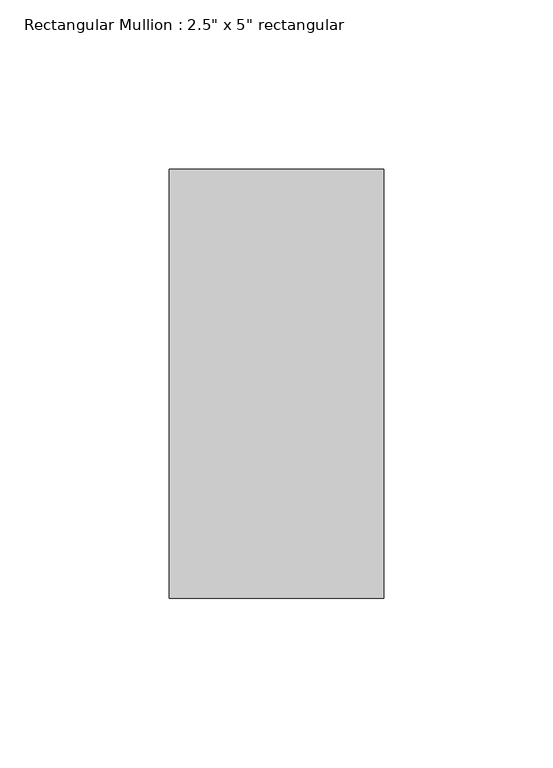
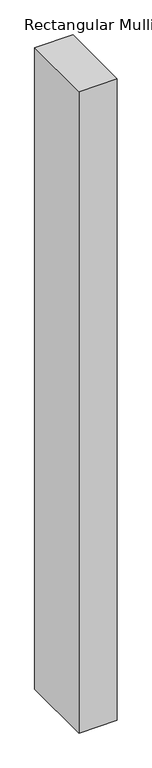
"""IFC4 building model written with IfcOpenShell, lengths in millimetres: member geometry."""

from ifc_helpers import new_model, si_unit, frame, origin, place, context, project, spatial, polyline, outline, extrude, source, transform, mapped, element, save


def member_d6c95716(model_context):
    return source(origin(), model_context, "Body", "SweptSolid", [
        extrude(outline(polyline([(0.0, 63.5), (0.0, -63.5), (-63.5, -63.5), (-63.5, 63.5), (0.0, 63.5)])), frame((0.0, 0.0, -1124.6130978), z_axis=(0.0, 0.0, 1.0), x_axis=(1.0, 0.0, 0.0)), (0.0, 0.0, 1.0), 1124.6130978),
    ])


if __name__ == "__main__":
    model = new_model("IFC4")
    model_context = context("Model", 3, world=origin())
    ifc_project = project(units=[si_unit("LENGTHUNIT", "METRE", prefix="MILLI")], contexts=[model_context])
    site = spatial("IfcSite", under=ifc_project)
    building = spatial("IfcBuilding", under=site)
    placement = place(None, origin())
    member_shape = member_d6c95716(model_context)
    element("IfcMember", 1, ObjectType="Rectangular Mullion : 2.5\" x 5\" rectangular", at=placement, inside=building, context=model_context, shape_type="MappedRepresentation", body=[
        mapped(member_shape, transform((0.0, 0.0, 0.0), x_axis=(1.0, 0.0, 0.0), y_axis=(0.0, 1.0, 0.0), z_axis=(0.0, 0.0, 1.0))),
    ])
    save(model, "model.ifc")

# Revit data of these elements
# Type "Rectangular Mullion : 2.5\" x 5\" rectangular"
#   built-in parameter 1007304 = 0.416667 (stored number, unit not read)
#   built-in parameter 1007301 = 0.104167 (stored number, unit not read)
#   built-in parameter 1007300 = 0.104167 (stored number, unit not read)
# Element 1 (IfcMember, "Rectangular Mullion : 2.5\" x 5\" rectangular")
#   Materials on its faces: "Aluminum"
# Materials
#   "Aluminum": class "Metal", colour RGB 247 247 247, transparency 0, Description = "Aluminum 6061", Cost = 0
